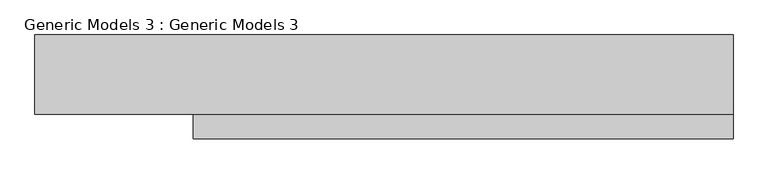
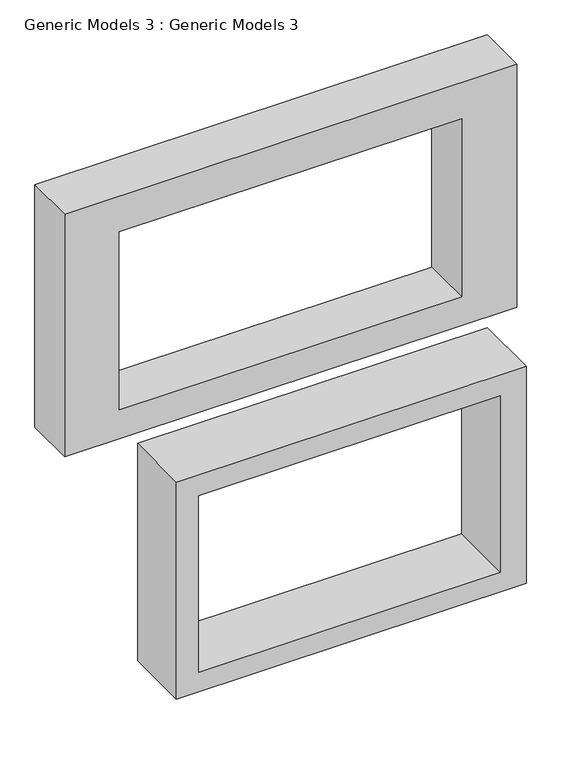
"""IFC4 building model written with IfcOpenShell, lengths in millimetres: proxy geometry, Generic Models 3 : Generic Models 3."""

from ifc_helpers import new_model, si_unit, frame, origin, place, context, project, spatial, polyline, outline, extrude, source, transform, mapped, element, save


def generic_models_3_generic_models_3_8d7ffd4d(model_context):
    return source(origin(), model_context, "Body", "SweptSolid", [
        extrude(outline(polyline([(2724.9812059, -5015.9403308), (2724.9812059, -9168.8403308), (0.0, -9168.8403308), (0.0, -5015.9403308), (2724.9812059, -5015.9403308)]), holes=[polyline([(241.8636012, -5319.8698177), (241.8636012, -8902.1403308), (2460.1511243, -8902.1403308), (2460.1511243, -5319.8698177), (241.8636012, -5319.8698177)])]), frame((0.0, -14153.4201119, 0.0), z_axis=(0.0, 1.0, 0.0), x_axis=(0.0, 0.0, 1.0)), (0.0, 0.0, 1.0), 798.0682381),
        extrude(outline(polyline([(6400.8, -5015.9403308), (6400.8, -10388.0403308), (3352.8, -10388.0403308), (3352.8, -5015.9403308), (6400.8, -5015.9403308)]), holes=[polyline([(5950.3309123, -5673.0510121), (3716.258733, -5673.0510121), (3716.258733, -9740.0667648), (5950.3309123, -9740.0667648), (5950.3309123, -5673.0510121)])]), frame((0.0, -13964.9518738, 0.0), z_axis=(0.0, 1.0, 0.0), x_axis=(0.0, 0.0, 1.0)), (0.0, 0.0, 1.0), 609.6),
    ])


if __name__ == "__main__":
    model = new_model("IFC4")
    model_context = context("Model", 3, world=origin())
    ifc_project = project(units=[si_unit("LENGTHUNIT", "METRE", prefix="MILLI")], contexts=[model_context])
    site = spatial("IfcSite", under=ifc_project)
    building = spatial("IfcBuilding", under=site)
    placement = place(None, origin())
    generic_models_3_generic_models_3_shape = generic_models_3_generic_models_3_8d7ffd4d(model_context)
    element("IfcBuildingElementProxy", 1, Name="Generic Models 3 : Generic Models 3", ObjectType="Generic Models 3 : Generic Models 3", at=placement, inside=building, context=model_context, shape_type="MappedRepresentation", body=[
        mapped(generic_models_3_generic_models_3_shape, transform((0.0, 0.0, 0.0), x_axis=(1.0, 0.0, 0.0), y_axis=(0.0, 1.0, 0.0), z_axis=(0.0, 0.0, 1.0))),
    ])
    save(model, "model.ifc")
